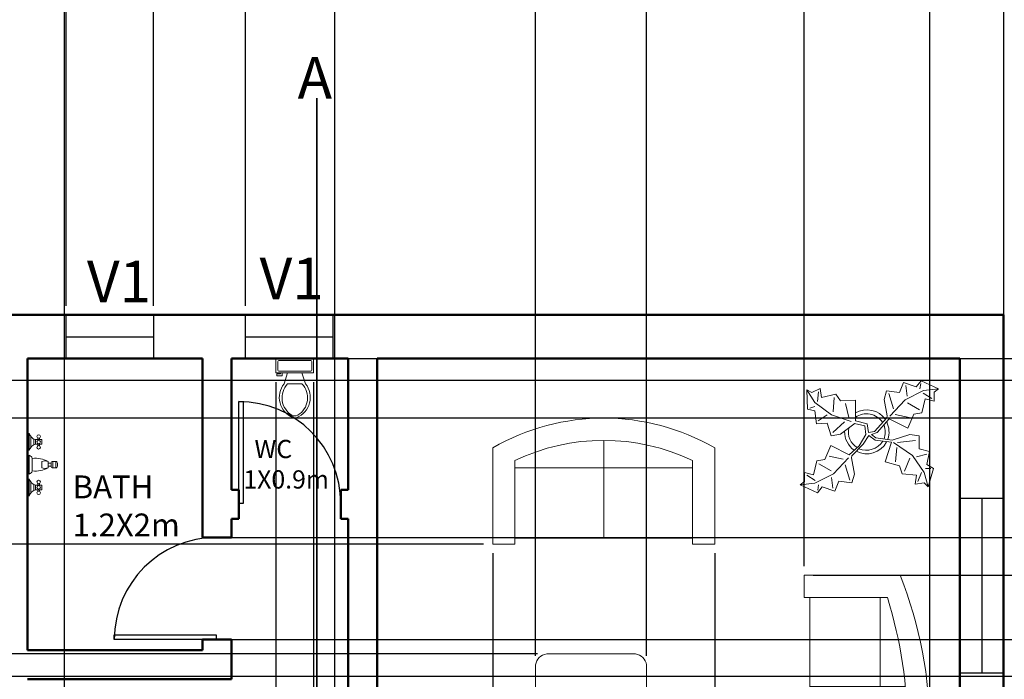
# Model space of a CAD drawing. Units: metres. Extents: x 2443.7 to 2482.9, y 2261.4 to 2287.
# Tile 5 of 8: x 2451.1 to 2457.9, y 2272.3 to 2276.8. Entities that reach past the tile are written whole.
import ezdxf

# ---------------------------------------------------------------- set-up
doc = ezdxf.new("R2010")
doc.units = ezdxf.units.M
for name, color, linetype, lineweight in [('A-ANNO-DIMS', 2, 'Continuous', 18), ('A-AREA-IDEN', 11, 'Continuous', 25), ('A-FLOR-FIXT', 20, 'Continuous', 18), ('A-MODL', 7, 'Continuous', 25), ('A-WALL', 7, 'Continuous', 50), ('door', 6, 'Continuous', 25), ('flower', 70, 'Continuous', 18), ('furnitures', 20, 'Continuous', 18), ('section', 1, 'Continuous', 35), ('text', 11, 'Continuous', 25), ('window', 3, 'Continuous', 25)]:
    doc.layers.add(name, color=color, linetype=linetype, lineweight=lineweight)
doc.styles.get("Standard").update_dxf_attribs({"font": 'arial.ttf'})
doc.dimstyles.get("Standard").update_dxf_attribs({"dimtxt": 0.18, "dimasz": 0.18, "dimexe": 0.18, "dimexo": 0.0625, "dimgap": 0.09, "dimtad": 0, "dimtih": 1, "dimtoh": 1, "dimdec": 4, "dimzin": 0, "dimdsep": 46, "dimtxsty": 'Standard', "dimcen": 0.09, "dimadec": 0, "dimazin": 0, "dimtfac": 1, "dimtdec": 4, "dimtofl": 0, "dimtmove": 0, "dimatfit": 3, "dimfxl": 1, "dimtolj": 1, "dimtzin": 0, "dimarcsym": 0})

# ---------------------------------------------------------------- blocks, each defined once
blk = doc.blocks.new('*U21')
for p, q in [((0, 0), (0, -6)), ((40, 0), (40, -6))]:
    blk.add_line(p, q)
blk.add_lwpolyline([(0, 0), (0, 40), (1.75, 40), (1.75, 0)], close=True)
blk.add_arc((0, 0), 40, 0, 90)
blk = doc.blocks.new('Plant - Rubber or Philodendron')
for p, q in [((8.8871, 10.7908), (9.9809, 13.4933)), ((9.9809, 13.4933), (13.3837, 12.301)), ((13.3837, 12.301), (14.68, 13.9039)), ((14.68, 13.9039), (19.3848, 11.8146)), ((-16.2005, 11.4774), (-13.9899, 8.1064)), ((-16.2005, 11.4774), (-14.8639, 10.7964)), ((-16.0159, 6.3329), (-16.2005, 11.4774)), ((-14.8639, 10.7964), (-12.6195, 11.8975)), ((-13.3174, 8.325), (-13.0735, 11.0065)), ((-12.6195, 11.8975), (-12.1909, 9.4345)), ((4.6914, 8.8812), (5.3859, 11.2828)), ((5.3859, 11.2828), (8.8871, 10.7908)), ((15.3859, 11.3055), (10.3916, 8.7942)), ((10.5828, 12.6946), (10.8893, 9.7953)), ((14.5816, 13.2037), (14.3848, 11.8033)), ((19.3848, 11.8146), (15.3859, 11.3055)), ((19.3848, 11.8146), (18.1868, 10.9119)), ((18.1868, 10.9119), (18.1925, 8.4119)), ((-13.9899, 8.1064), (-9.5434, 4.7185)), ((-12.1909, 9.4345), (-8.3829, 10.3)), ((-8.8369, 9.409), (-9.0894, 5.6095)), ((-8.3829, 10.3), (-7.0549, 8.501)), ((-7.0549, 8.501), (-3.0284, 8.6941)), ((-3.0284, 8.6941), (-3.0709, 3.1041)), ((4.6914, 8.8812), (5.5014, 4.4831)), ((5.9878, 10.4842), (7.1971, 6.3869)), ((10.3916, 8.7942), (6.2847, 4.4028)), ((14.2977, 6.1031), (10.9934, 7.9956)), ((15.7909, 9.1065), (14.8995, 5.3044)), ((15.2875, 10.6053), (17.5907, 9.2105)), ((18.1925, 8.4119), (15.7909, 9.1065)), ((-14.0069, 5.8704), (-16.0159, 6.3329)), ((-15.3434, 6.5514), (-13.9984, 6.9884)), ((-13.5868, 2.2894), (-14.0069, 5.8704)), ((-4.8529, 4.012), (-5.7184, 7.82)), ((-13.1329, 3.1804), (-10.6614, 4.727)), ((-9.5434, 4.7185), (-4.1917, 2.9888)), ((-9.1318, 0.0195), (-5.9793, 2.9025)), ((-3.0709, 3.1041), (0.0797, 2.3163)), ((2.1141, 0.2298), (5.4346, 3.9146)), ((6.1032, 3.6844), (2.8262, -0.031)), ((5.4346, 3.9146), (5.5014, 4.4831)), ((11.1089, 1.1958), (6.1032, 3.6844)), ((7.7005, 4.8881), (11.5025, 3.9967)), ((12.7005, 4.8994), (11.1089, 1.1958)), ((14.8995, 5.3044), (12.7005, 4.8994)), ((-10.6784, 2.491), (-13.5868, 2.2894)), ((-9.5858, -0.8715), (-10.6784, 2.491)), ((-7.1228, -0.443), (-3.5248, 2.2131)), ((-3.5248, 2.2131), (-3.3011, 2.4355)), ((-3.3011, 2.4355), (-0.5306, 1.7947)), ((-0.5306, 1.7947), (-0.2255, -0.5527)), ((-0.5306, 1.7947), (-0.5306, 1.7947)), ((0.0797, 2.3163), (0.4866, -0.031)), ((0.4866, -0.031), (2.1141, 0.2298)), ((-7.1228, -0.443), (-9.5858, -0.8715)), ((-2.019, -3.6148), (-0.2255, -0.5527)), ((-0.9375, -3.1608), (0.5883, -0.8135)), ((0.5883, -0.8135), (2.2447, -2.0916)), ((2.8262, -0.031), (1.3003, -0.5527)), ((1.3003, -0.5527), (2.4193, -1.4655)), ((2.2447, -2.0916), (6.7108, -2.6626)), ((2.4193, -1.4655), (6.895, -2.1175)), ((11.6605, -0.5413), (6.895, -2.1175)), ((8.3544, -2.7453), (13.1973, -2.1704)), ((11.6605, -0.5413), (14.1354, -0.8948)), ((14.1354, -0.8948), (14.1354, -4.4304)), ((-11.3237, -7.2629), (-9.7321, -3.5593)), ((-9.7321, -3.5593), (-4.7264, -6.0479)), ((-2.019, -3.6148), (-4.7264, -6.0479)), ((-4.0579, -6.2781), (-0.9375, -3.1608)), ((4.943, -7.9659), (6.7108, -2.6626)), ((12.3677, -6.1981), (7.219, -2.6772)), ((8.125, -4.0768), (7.7715, -7.9659)), ((14.1354, -4.4304), (16.9638, -5.1375)), ((16.9638, -5.1375), (16.2567, -8.673)), ((-14.4141, -11.4699), (-13.5228, -7.6679)), ((-13.5228, -7.6679), (-11.3237, -7.2629)), ((-6.3237, -7.2516), (-10.1257, -6.3602)), ((-9.0148, -11.1577), (-4.9047, -6.8122)), ((-4.1246, -6.8466), (-4.0579, -6.2781)), ((-3.3146, -11.2447), (-4.1246, -6.8466)), ((8.8321, -9.0266), (4.943, -7.9659)), ((10.2463, -10.4408), (11.6605, -6.9053)), ((15.5496, -10.7943), (12.3677, -6.1981)), ((16.2567, -5.8446), (13.4283, -6.5517)), ((-12.921, -8.4665), (-9.6166, -10.359)), ((-4.611, -12.8477), (-5.8203, -8.7504)), ((9.5392, -11.1479), (8.8321, -9.0266)), ((17.3174, -9.7337), (15.9032, -9.7337)), ((16.2567, -8.673), (18.0245, -9.7337)), ((18.0245, -9.7337), (16.6103, -14.6834)), ((-18.008, -14.1781), (-16.8101, -13.2754)), ((-16.8157, -10.7754), (-14.4141, -11.4699)), ((-16.8101, -13.2754), (-16.8157, -10.7754)), ((-13.9107, -12.9688), (-16.2139, -11.574)), ((-14.0091, -13.669), (-9.0148, -11.1577)), ((-9.206, -15.0581), (-9.5126, -12.1588)), ((-7.5103, -13.1543), (-8.6042, -15.8568)), ((-4.0092, -13.6463), (-7.5103, -13.1543)), ((-3.3146, -11.2447), (-4.0092, -13.6463)), ((13.4283, -11.5015), (9.5392, -11.1479)), ((13.0748, -13.9763), (13.4283, -11.5015)), ((14.8425, -10.7943), (13.7819, -13.2692)), ((16.6103, -14.6834), (15.5496, -10.7943)), ((-18.008, -14.1781), (-14.0091, -13.669)), ((-13.3032, -16.2674), (-18.008, -14.1781)), ((-12.0069, -14.6645), (-13.3032, -16.2674)), ((-13.2048, -15.5672), (-13.008, -14.1668)), ((-8.6042, -15.8568), (-12.0069, -14.6645)), ((15.5496, -13.6228), (13.0748, -13.9763)), ((16.6103, -14.6834), (15.5496, -13.6228))]:
    blk.add_line(p, q)
for centre, radius, start, end in [((0, 0), 6.1275, 34.37569, 120.1028), ((-0.0601, -0.2075), 5.2461, 33.82192, 124.9414), ((-0.098, 0.1364), 6.1288, 341.2017, 26.09184), ((0.0308, 0.1664), 6, 178.6147, 235.1169), ((0.0308, 0.1664), 5, 168.1647, 238.6725), ((-0.2664, 0.1682), 5.2775, 338.4094, 20.03007), ((-0.0234, 0.3825), 6.1492, 242.5812, 331.2714), ((-0.1102, 0.4886), 5.2883, 247.3711, 327.472)]:
    blk.add_arc(centre, radius, start, end)
blk = doc.blocks.new('Sofa - Roundback 7 ft.')
for p, q in [((-12.00002, -32.4421), (-12.00003, -6.5971)), ((11.99997, -32.4421), (11.99998, -6.5971)), ((-36.000027, -34), (-36.000027, -11.4696)), ((35.99998, -34), (35.99998, -11.4696)), ((-35.999844, -13.3819), (35.9998, -13.3819)), ((-36.000027, -32.4421), (35.99998, -32.4421))]:
    blk.add_line(p, q)
for points in [[(-36.000027, -34), (-42.000027, -34), (-42.000027, -8)], [(41.99998, -8), (41.99998, -34), (35.99998, -34)]]:
    blk.add_lwpolyline(points)
for centre, radius, start, end in [((0, -114.25), 114.25, 68.43141, 111.5686), ((-0.00001, -127.1968), 121.1968, 72.72033, 107.2797)]:
    blk.add_arc(centre, radius, start, end)
blk = doc.blocks.new('Sofa - Roundback Loveseat 5 ft.')
for p, q in [((0, -32.44198), (0, -5.99998)), ((-24, -33.99998), (-24, -11.46958)), ((24.00004, -33.99998), (24.00004, -11.46958)), ((-23.9998, -13.38178), (23.99986, -13.38178)), ((-24, -32.44198), (24.00004, -32.44198))]:
    blk.add_line(p, q)
for points in [[(-24, -33.99998), (-30, -33.99998), (-30, -7.99998)], [(30.00004, -7.99998), (30.00004, -33.99998), (24.00004, -33.99998)]]:
    blk.add_lwpolyline(points)
for centre, radius, start, end in [((0, -60.24998), 60.24998, 60.13715, 119.8628), ((0, -61.38438), 55.38444, 64.32083, 115.6792)]:
    blk.add_arc(centre, radius, start, end)
blk = doc.blocks.new('Desk - 30 x 60 in.')
for p, q in [((-26.999995, 0), (26.999995, 0)), ((-29.999995, -27), (-29.999995, -3)), ((29.999995, -3), (29.999995, -27)), ((26.999995, -30), (-26.999995, -30)), ((-20.000005, -30), (-20.000005, -31)), ((-20.000005, -31), (-16.000005, -31)), ((-16.000005, -31), (-16.000005, -30)), ((15.999995, -31), (15.999995, -30)), ((19.999995, -31), (15.999995, -31)), ((19.999995, -30), (19.999995, -31))]:
    blk.add_line(p, q)
for centre, start, end in [((-26.499995, -3.5), 98.1301, 171.8699), ((26.499995, -3.5), 8.130102, 81.8699), ((-26.499995, -26.5), 188.1301, 261.8699), ((26.499995, -26.5), 278.1301, 351.8699)]:
    blk.add_arc(centre, 3.535534, start, end)
blk = doc.blocks.new('Toilet - top')
for p, q in [((9.5, -6), (9.5, -2)), ((-10, -8.5), (-8, -8.5)), ((-10, -9.5), (-10, -8.5)), ((-7, -9.5), (-10, -9.5)), ((-8, -8.5), (-8, -8)), ((-7, -8), (-7, -9.5)), ((-4, -8), (-6, -14)), ((4, -8), (6, -14)), ((4, -14), (-4, -14))]:
    blk.add_line(p, q)
blk.add_lwpolyline([(10.5, -8), (10.5, 0), (-10.5, 0), (-10.5, -8)], close=True)
for points in [[(-9.5, -2), (-9.5, -6)], [(8.5, -1), (-8.5, -1)], [(-8.5, -7), (8.5, -7)]]:
    blk.add_lwpolyline(points)
for centre, radius, start, end in [((-8.62, -1.88), 0.884, 81.8699, 188.1301), ((8.62, -1.88), 0.884, 351.8699, 98.1301), ((-8.62, -6.12), 0.884, 171.8699, 278.1301), ((8.62, -6.12), 0.884, 261.8699, 8.1301), ((3.52, -21.58), 12.17, 141.4691, 247.9714), ((4.2, -21.82), 11.33, 136.3677, 238.9468), ((-3.52, -21.58), 12.17, 292.0284, 38.5307), ((-4.2, -21.82), 11.33, 301.053, 43.6321), ((0, -27.88), 4, 245.7318, 294.2682), ((0, -29), 4, 254.8605, 285.1395)]:
    blk.add_arc(centre, radius, start, end)
blk = doc.blocks.new('Faucet - Bathroom front')
for p, q in [((-0.5, 4.25), (0.5, 4.25)), ((0.5, 3.75), (-0.5, 3.75)), ((-0.25, 3), (-0.25, 3.5)), ((0.25, 3.5), (0.25, 3)), ((-4, 1.625), (-4.25, 1.625)), ((-3.25, 1.625), (-3, 1.625)), ((-0.5, 3), (0.5, 3)), ((0.5, 2), (-0.5, 2)), ((3.25, 1.625), (3, 1.625)), ((4, 1.625), (4.25, 1.625)), ((-5, 0), (-2.25, 0)), ((-4.5087, 0.25), (-2.7408, 0.25)), ((-4, 1.375), (-4.25, 1.375)), ((-3.1442, 0.75), (-4.0979, 0.75)), ((-3.25, 1.375), (-3, 1.375)), ((-1.5, 0), (1.5, 0)), ((-1, 0.5), (1, 0.5)), ((2.25, 0), (5, 0)), ((2.7413, 0.25), (4.5092, 0.25)), ((3.25, 1.375), (3, 1.375)), ((4.1058, 0.75), (3.1521, 0.75)), ((4, 1.375), (4.25, 1.375))]:
    blk.add_line(p, q)
for points in [[(-0.5, 3.75), (-0.5, 4.25)], [(-0.25, 4.5), (0.25, 4.5)], [(0.25, 3.5), (-0.25, 3.5)], [(0.5, 4.25), (0.5, 3.75)]]:
    blk.add_lwpolyline(points)
for points in [[(-4, 1), (-4, 2), (-3.25, 2), (-3.25, 1)], [(3.25, 1), (3.25, 2), (4, 2), (4, 1)]]:
    blk.add_lwpolyline(points, close=True)
for centre in [(-4.5, 1.5), (-3.625, 1.5), (-2.75, 1.5), (2.75, 1.5), (3.625, 1.5), (4.5, 1.5)]:
    blk.add_circle(centre, 0.2795)
for centre, radius, start, end in [((-0.2575, 4.2575), 0.2426, 88.22243, 181.7776), ((-0.2575, 3.7425), 0.2426, 178.2224, 271.7776), ((0.2575, 4.2575), 0.2426, 358.2224, 91.77757), ((0.2575, 3.7425), 0.2426, 268.2224, 1.777565), ((3, 1), 4.0311, 150.2551, 187.125), ((0.6413, 2.5), 1.246, 156.3417, 203.6583), ((-3, 1), 4.0311, 352.875, 29.74488), ((-0.6413, 2.5), 1.246, 336.3417, 23.65835), ((-5.375, 1.375), 1.4252, 285.2551, 344.7449), ((-1.875, 1.375), 1.4252, 195.2551, 254.7449), ((-0.7962, -0.2038), 0.7327, 106.1502, 163.8498), ((0.7962, -0.2038), 0.7327, 16.1502, 73.84979), ((1.875, 1.375), 1.4252, 285.2551, 344.7449), ((5.375, 1.375), 1.4252, 195.2551, 254.7449)]:
    blk.add_arc(centre, radius, start, end)
blk = doc.blocks.new('aditya')
at = {"layer": 'A-WALL'}
for p, q in [((0, 9.9), (10.2, 9.9)), ((10.2, 3.3), (10.2, 9.9)), ((3.5, 7.6), (3.5, 9.6)), ((3.5, 9.6), (4.7, 9.6)), ((4.7, 8.3734), (4.7, 9.6)), ((4.9, 8.7), (4.9, 9.6)), ((4.9, 9.6), (5.7, 9.6)), ((5.7, 8.7), (5.7, 9.6)), ((5.9, 6.0521), (5.9, 9.6)), ((5.9, 9.6), (9.9, 9.6)), ((9.9, 5), (9.9, 9.6)), ((4.9, 8.7), (4.9503, 8.7)), ((5.6503, 8.7), (5.7, 8.7)), ((4.9, 8.3734), (4.9, 8.5)), ((4.9, 8.5), (4.9503, 8.5)), ((5.6503, 8.5), (5.7, 8.5)), ((5.7, 6.0521), (5.7, 8.5)), ((4.7, 7.6), (4.7, 7.6734)), ((4.9, 7.4), (4.9, 7.6734)), ((3.5, 7.6), (4.7, 7.6)), ((3.5, 7.4), (4.9, 7.4))]:
    blk.add_line(p, q, dxfattribs=at)
for points in [[(4.9503, 8.5), (4.9503, 8.7)], [(5.6503, 8.7), (5.6503, 8.5)], [(4.7, 8.3734), (4.9, 8.3734)], [(4.9, 7.6734), (4.7, 7.6734)]]:
    blk.add_lwpolyline(points, dxfattribs=at)
at = {"layer": 'section'}
blk.add_line((5.4866, -1.5581), (5.4866, 11.3875), dxfattribs=at)
at = {"layer": 'window'}
for p, q in [((3.7644, 9.75), (4.3644, 9.75)), ((4.9948, 9.75), (5.5948, 9.75)), ((10.05, 8.642), (10.05, 7.442))]:
    blk.add_line(p, q, dxfattribs=at)
for points in [[(3.7644, 9.6), (3.7644, 9.9), (4.3644, 9.9), (4.3644, 9.6)], [(4.9948, 9.6), (4.9948, 9.9), (5.5948, 9.9), (5.5948, 9.6)], [(9.9, 8.642), (10.2, 8.642), (10.2, 7.442), (9.9, 7.442)]]:
    blk.add_lwpolyline(points, close=True, dxfattribs=at)
at = {"layer": 'A-FLOR-FIXT', "xscale": 0.0123151634342974, "yscale": 0.0123151634342974, "zscale": 0.0123151634342974}
blk.add_blockref('Toilet - top', (5.3344, 9.6), dxfattribs=at)
at = {"layer": 'A-FLOR-FIXT', "xscale": 0.0430474379416969, "yscale": 0.0430474379416969, "zscale": 0.0430474379416969, "rotation": 270}
blk.add_blockref('Faucet - Bathroom front', (3.511, 8.8725), dxfattribs=at)
at = {"layer": 'door', "xscale": 0.0174999999999987, "yscale": 0.0174999999999987, "zscale": 0.0174999999999987}
blk.add_blockref('*U21', (4.9503, 8.605), dxfattribs=at)
at = {"layer": 'door', "xscale": 0.0174999999999987, "yscale": 0.0174999999999987, "zscale": 0.0174999999999987, "rotation": 90}
blk.add_blockref('*U21', (4.795, 7.6734), dxfattribs=at)
at = {"layer": 'flower', "xscale": 0.0254, "yscale": 0.0254, "zscale": 0.0254}
blk.add_blockref('Plant - Rubber or Philodendron', (9.2606, 9.0935), dxfattribs=at)
at = {"layer": 'furnitures', "xscale": 0.0254, "yscale": 0.0254, "zscale": 0.0254}
blk.add_blockref('Sofa - Roundback Loveseat 5 ft.', (7.4549, 9.1917), dxfattribs=at)
for name, p, rotation in [('Sofa - Roundback 7 ft.', (9.6938, 7.0466), 270), ('Desk - 30 x 60 in.', (6.9873, 6.8124), 90)]:
    blk.add_blockref(name, p, dxfattribs=dict(at, rotation=rotation))
at = {"layer": 'A-AREA-IDEN', "attachment_point": 1}
for s, width, gutter_width, insert, char_height in [('{\\fArial|b1|i1|c0|p34;  WC\\P1X0.9m}', 5.273298, 3.9123, (4.9809, 9.0426), 0.125192), ('{\\fArial|b1|i1|c0|p34;BATH\\P1.2X2m}', 6.599358, 4.8961, (3.8093, 8.7984), 0.156674)]:
    blk.add_mtext_dynamic_manual_height_columns(s, width=width, gutter_width=gutter_width, heights=[0], dxfattribs=dict(at, insert=insert, char_height=char_height))
at = {"layer": 'text'}
for s, height, p in [('A', 0.2853, (5.3535, 11.3838)), ('V1', 0.28528, (5.0929, 10.0065)), ('V1', 0.28528, (3.9077, 9.9863))]:
    blk.add_text(s, height=height, dxfattribs=at).set_placement(p)
blk = doc.blocks.new('*D23')
at = {"layer": 'A-ANNO-DIMS', "color": 0, "lineweight": -2, "transparency": 16777216}
for p, q in [((2457.9453, 2274.7597), (2482.2428, 2274.7597)), ((2482.0628, 2274.5797), (2482.0628, 2269.6416)), ((2482.0628, 2264.3397), (2482.0628, 2269.2778)), ((2453.6453, 2264.1597), (2482.2428, 2264.1597))]:
    blk.add_line(p, q, dxfattribs=at)
at = {"layer": 'A-ANNO-DIMS', "color": 0, "transparency": 16777216}
for points in [[(2482.0328, 2274.5797), (2482.0928, 2274.5797), (2482.0628, 2274.7597)], [(2482.0328, 2264.3397), (2482.0928, 2264.3397), (2482.0628, 2264.1597)]]:
    blk.add_solid(points, dxfattribs=at)
at = {"layer": 'Defpoints', "color": 0, "transparency": 16777216}
for p in [(2457.8828, 2274.7597), (2453.5828, 2264.1597), (2482.0628, 2264.1597)]:
    blk.add_point(p, dxfattribs=at)
at = {"layer": 'A-ANNO-DIMS', "color": 0, "transparency": 16777216, "insert": (2482.0628, 2269.4597), "char_height": 0.18, "attachment_point": 5}
blk.add_mtext('\\A1;10.6', dxfattribs=at)
blk = doc.blocks.new('*D28')
at = {"layer": 'A-ANNO-DIMS', "color": 0, "lineweight": -2, "transparency": 16777216}
for p, q in [((2449.9171, 2274.8222), (2449.9171, 2287.0152)), ((2451.4471, 2274.8222), (2451.4471, 2287.0152)), ((2450.0971, 2286.8352), (2450.3668, 2286.8352)), ((2451.2671, 2286.8352), (2450.9974, 2286.8352))]:
    blk.add_line(p, q, dxfattribs=at)
at = {"layer": 'A-ANNO-DIMS', "color": 0, "transparency": 16777216}
for points in [[(2450.0971, 2286.8652), (2450.0971, 2286.8052), (2449.9171, 2286.8352)], [(2451.2671, 2286.8652), (2451.2671, 2286.8052), (2451.4471, 2286.8352)]]:
    blk.add_solid(points, dxfattribs=at)
at = {"layer": 'Defpoints', "color": 0, "transparency": 16777216}
for p in [(2451.4471, 2286.8352), (2449.9171, 2274.7597), (2451.4471, 2274.7597)]:
    blk.add_point(p, dxfattribs=at)
at = {"layer": 'A-ANNO-DIMS', "color": 0, "transparency": 16777216, "insert": (2450.6821, 2286.8352), "char_height": 0.18, "attachment_point": 5}
blk.add_mtext('\\A1;1.53', dxfattribs=at)
blk = doc.blocks.new('*D29')
at = {"layer": 'A-ANNO-DIMS', "color": 0, "lineweight": -2, "transparency": 16777216}
for p, q in [((2451.4471, 2274.8222), (2451.4471, 2287.0152)), ((2452.0471, 2274.8222), (2452.0471, 2287.0152)), ((2451.6271, 2286.8352), (2451.8671, 2286.8352)), ((2452.0471, 2286.8352), (2452.2271, 2286.8352))]:
    blk.add_line(p, q, dxfattribs=at)
at = {"layer": 'A-ANNO-DIMS', "color": 0, "transparency": 16777216}
for points in [[(2451.6271, 2286.8652), (2451.6271, 2286.8052), (2451.4471, 2286.8352)], [(2451.8671, 2286.8652), (2451.8671, 2286.8052), (2452.0471, 2286.8352)]]:
    blk.add_solid(points, dxfattribs=at)
at = {"layer": 'Defpoints', "color": 0, "transparency": 16777216}
for p in [(2452.0471, 2286.8352), (2451.4471, 2274.7597), (2452.0471, 2274.7597)]:
    blk.add_point(p, dxfattribs=at)
at = {"layer": 'A-ANNO-DIMS', "color": 0, "transparency": 16777216, "insert": (2452.4809, 2286.8352), "char_height": 0.18, "attachment_point": 5}
blk.add_mtext('\\A1;0.6', dxfattribs=at)
blk = doc.blocks.new('*D30')
at = {"layer": 'A-ANNO-DIMS', "color": 0, "lineweight": -2, "transparency": 16777216}
for p, q in [((2452.0471, 2274.8222), (2452.0471, 2287.0152)), ((2452.6776, 2274.8222), (2452.6776, 2287.0152)), ((2452.2271, 2286.8352), (2452.4976, 2286.8352)), ((2452.6776, 2286.8352), (2452.8576, 2286.8352))]:
    blk.add_line(p, q, dxfattribs=at)
at = {"layer": 'A-ANNO-DIMS', "color": 0, "transparency": 16777216}
for points in [[(2452.2271, 2286.8652), (2452.2271, 2286.8052), (2452.0471, 2286.8352)], [(2452.4976, 2286.8652), (2452.4976, 2286.8052), (2452.6776, 2286.8352)]]:
    blk.add_solid(points, dxfattribs=at)
at = {"layer": 'Defpoints', "color": 0, "transparency": 16777216}
for p in [(2452.6776, 2286.8352), (2452.0471, 2274.7597), (2452.6776, 2274.7597)]:
    blk.add_point(p, dxfattribs=at)
at = {"layer": 'A-ANNO-DIMS', "color": 0, "transparency": 16777216, "insert": (2453.1813, 2286.8352), "char_height": 0.18, "attachment_point": 5}
blk.add_mtext('\\A1;0.63', dxfattribs=at)
blk = doc.blocks.new('*D34')
at = {"layer": 'A-ANNO-DIMS', "color": 0, "lineweight": -2, "transparency": 16777216}
for p, q in [((2457.9453, 2274.7597), (2482.2428, 2274.7597)), ((2482.0628, 2274.5797), (2482.0628, 2274.3126)), ((2482.0628, 2273.6817), (2482.0628, 2273.9488)), ((2457.9453, 2273.5017), (2482.2428, 2273.5017))]:
    blk.add_line(p, q, dxfattribs=at)
at = {"layer": 'A-ANNO-DIMS', "color": 0, "transparency": 16777216}
for points in [[(2482.0328, 2274.5797), (2482.0928, 2274.5797), (2482.0628, 2274.7597)], [(2482.0328, 2273.6817), (2482.0928, 2273.6817), (2482.0628, 2273.5017)]]:
    blk.add_solid(points, dxfattribs=at)
at = {"layer": 'Defpoints', "color": 0, "transparency": 16777216}
for p in [(2457.8828, 2274.7597), (2457.8828, 2273.5017), (2482.0628, 2273.5017)]:
    blk.add_point(p, dxfattribs=at)
at = {"layer": 'A-ANNO-DIMS', "color": 0, "transparency": 16777216, "insert": (2482.0628, 2274.1307), "char_height": 0.18, "attachment_point": 5}
blk.add_mtext('\\A1;1.258', dxfattribs=at)
blk = doc.blocks.new('*D35')
at = {"layer": 'A-ANNO-DIMS', "color": 0, "lineweight": -2, "transparency": 16777216}
for p, q in [((2457.9453, 2272.3017), (2482.2428, 2272.3017)), ((2482.0628, 2272.1217), (2482.0628, 2271.6247)), ((2482.0628, 2270.7669), (2482.0628, 2271.2639)), ((2457.9453, 2270.5869), (2482.2428, 2270.5869))]:
    blk.add_line(p, q, dxfattribs=at)
at = {"layer": 'A-ANNO-DIMS', "color": 0, "transparency": 16777216}
for points in [[(2482.0328, 2272.1217), (2482.0928, 2272.1217), (2482.0628, 2272.3017)], [(2482.0328, 2270.7669), (2482.0928, 2270.7669), (2482.0628, 2270.5869)]]:
    blk.add_solid(points, dxfattribs=at)
at = {"layer": 'Defpoints', "color": 0, "transparency": 16777216}
for p in [(2457.8828, 2272.3017), (2457.8828, 2270.5869), (2482.0628, 2270.5869)]:
    blk.add_point(p, dxfattribs=at)
at = {"layer": 'A-ANNO-DIMS', "color": 0, "transparency": 16777216, "insert": (2482.0628, 2271.4443), "char_height": 0.18, "attachment_point": 5}
blk.add_mtext('\\A1;1.71', dxfattribs=at)
blk = doc.blocks.new('*D37')
at = {"layer": 'A-ANNO-DIMS', "color": 0, "lineweight": -2, "transparency": 16777216}
for p, q in [((2450.1874, 2274.3123), (2482.2428, 2274.3123)), ((2482.0628, 2274.1323), (2482.0628, 2273.4783)), ((2482.0628, 2272.4603), (2482.0628, 2273.1144)), ((2450.1874, 2272.2803), (2482.2428, 2272.2803))]:
    blk.add_line(p, q, dxfattribs=at)
at = {"layer": 'A-ANNO-DIMS', "color": 0, "transparency": 16777216}
for points in [[(2482.0328, 2274.1323), (2482.0928, 2274.1323), (2482.0628, 2274.3123)], [(2482.0328, 2272.4603), (2482.0928, 2272.4603), (2482.0628, 2272.2803)]]:
    blk.add_solid(points, dxfattribs=at)
at = {"layer": 'Defpoints', "color": 0, "transparency": 16777216}
for p in [(2450.1249, 2274.3123), (2482.0628, 2274.3123), (2450.1249, 2272.2803)]:
    blk.add_point(p, dxfattribs=at)
at = {"layer": 'A-ANNO-DIMS', "color": 0, "transparency": 16777216, "insert": (2482.0628, 2273.2963), "char_height": 0.18, "attachment_point": 5}
blk.add_mtext('\\A1;2.032', dxfattribs=at)
blk = doc.blocks.new('*D38')
at = {"layer": 'A-ANNO-DIMS', "color": 0, "lineweight": -2, "transparency": 16777216}
for p, q in [((2454.3757, 2273.1253), (2454.3757, 2261.3876)), ((2455.8997, 2273.1253), (2455.8997, 2261.3876)), ((2454.5557, 2261.5676), (2454.7528, 2261.5676)), ((2455.7197, 2261.5676), (2455.5225, 2261.5676))]:
    blk.add_line(p, q, dxfattribs=at)
at = {"layer": 'A-ANNO-DIMS', "color": 0, "transparency": 16777216}
for points in [[(2454.5557, 2261.5976), (2454.5557, 2261.5376), (2454.3757, 2261.5676)], [(2455.7197, 2261.5976), (2455.7197, 2261.5376), (2455.8997, 2261.5676)]]:
    blk.add_solid(points, dxfattribs=at)
at = {"layer": 'Defpoints', "color": 0, "transparency": 16777216}
for p in [(2454.3757, 2273.1878), (2455.8997, 2273.1878), (2454.3757, 2261.5676)]:
    blk.add_point(p, dxfattribs=at)
at = {"layer": 'A-ANNO-DIMS', "color": 0, "transparency": 16777216, "insert": (2455.1377, 2261.5676), "char_height": 0.18, "attachment_point": 5}
blk.add_mtext('\\A1;1.524', dxfattribs=at)
blk = doc.blocks.new('*D39')
at = {"layer": 'A-ANNO-DIMS', "color": 0, "lineweight": -2, "transparency": 16777216}
for p, q in [((2444.2827, 2274.0514), (2444.2827, 2274.2314)), ((2444.2827, 2274.2314), (2444.4627, 2274.2314)), ((2455.0752, 2274.0514), (2444.1027, 2274.0514)), ((2444.2827, 2273.3678), (2444.2827, 2273.8714)), ((2454.3132, 2273.1878), (2444.1027, 2273.1878))]:
    blk.add_line(p, q, dxfattribs=at)
at = {"layer": 'A-ANNO-DIMS', "color": 0, "transparency": 16777216}
for points in [[(2444.2527, 2273.8714), (2444.3127, 2273.8714), (2444.2827, 2274.0514)], [(2444.2527, 2273.3678), (2444.3127, 2273.3678), (2444.2827, 2273.1878)]]:
    blk.add_solid(points, dxfattribs=at)
at = {"layer": 'Defpoints', "color": 0, "transparency": 16777216}
for p in [(2444.2827, 2274.0514), (2455.1377, 2274.0514), (2454.3757, 2273.1878)]:
    blk.add_point(p, dxfattribs=at)
at = {"layer": 'A-ANNO-DIMS', "color": 0, "transparency": 16777216, "insert": (2444.7864, 2274.2314), "char_height": 0.18, "attachment_point": 5}
blk.add_mtext('\\A1;0.86', dxfattribs=at)
blk = doc.blocks.new('*D40')
at = {"layer": 'A-ANNO-DIMS', "color": 0, "lineweight": -2, "transparency": 16777216}
for p, q in [((2456.5754, 2272.973), (2482.2428, 2272.973)), ((2482.0628, 2272.793), (2482.0628, 2272.0882)), ((2482.0628, 2271.0194), (2482.0628, 2271.7243)), ((2456.5754, 2270.8394), (2482.2428, 2270.8394))]:
    blk.add_line(p, q, dxfattribs=at)
at = {"layer": 'A-ANNO-DIMS', "color": 0, "transparency": 16777216}
for points in [[(2482.0328, 2272.793), (2482.0928, 2272.793), (2482.0628, 2272.973)], [(2482.0328, 2271.0194), (2482.0928, 2271.0194), (2482.0628, 2270.8394)]]:
    blk.add_solid(points, dxfattribs=at)
at = {"layer": 'Defpoints', "color": 0, "transparency": 16777216}
for p in [(2456.5129, 2272.973), (2482.0628, 2272.973), (2456.5129, 2270.8394)]:
    blk.add_point(p, dxfattribs=at)
at = {"layer": 'A-ANNO-DIMS', "color": 0, "transparency": 16777216, "insert": (2482.0628, 2271.9062), "char_height": 0.18, "attachment_point": 5}
blk.add_mtext('\\A1;2.13', dxfattribs=at)
blk = doc.blocks.new('*D41')
at = {"layer": 'A-ANNO-DIMS', "color": 0, "lineweight": -2, "transparency": 16777216}
for p, q in [((2456.512931, 2273.035548), (2456.512931, 2287.015188)), ((2457.376531, 2271.968748), (2457.376531, 2287.015188)), ((2456.332931, 2286.835188), (2456.152931, 2286.835188)), ((2457.556531, 2286.835188), (2457.736531, 2286.835188))]:
    blk.add_line(p, q, dxfattribs=at)
at = {"layer": 'A-ANNO-DIMS', "color": 0, "transparency": 16777216}
for points in [[(2456.332931, 2286.865188), (2456.332931, 2286.805188), (2456.512931, 2286.835188)], [(2457.556531, 2286.865188), (2457.556531, 2286.805188), (2457.376531, 2286.835188)]]:
    blk.add_solid(points, dxfattribs=at)
at = {"layer": 'Defpoints', "color": 0, "transparency": 16777216}
for p in [(2457.376531, 2286.835188), (2456.512931, 2272.973048), (2457.376531, 2271.906248)]:
    blk.add_point(p, dxfattribs=at)
at = {"layer": 'A-ANNO-DIMS', "color": 0, "transparency": 16777216, "insert": (2456.944731, 2286.835188), "char_height": 0.18, "attachment_point": 5}
blk.add_mtext('\\A1;0.86', dxfattribs=at)
blk = doc.blocks.new('*D42')
at = {"layer": 'A-ANNO-DIMS', "color": 0, "lineweight": -2, "transparency": 16777216}
for p, q in [((2454.6838, 2272.434), (2444.1027, 2272.434)), ((2444.2827, 2272.254), (2444.2827, 2271.854)), ((2444.2827, 2271.09), (2444.2827, 2271.4901)), ((2454.6838, 2270.91), (2444.1027, 2270.91))]:
    blk.add_line(p, q, dxfattribs=at)
at = {"layer": 'A-ANNO-DIMS', "color": 0, "transparency": 16777216}
for points in [[(2444.2527, 2272.254), (2444.3127, 2272.254), (2444.2827, 2272.434)], [(2444.2527, 2271.09), (2444.3127, 2271.09), (2444.2827, 2270.91)]]:
    blk.add_solid(points, dxfattribs=at)
at = {"layer": 'Defpoints', "color": 0, "transparency": 16777216}
for p in [(2444.2827, 2272.434), (2454.7463, 2272.434), (2454.7463, 2270.91)]:
    blk.add_point(p, dxfattribs=at)
at = {"layer": 'A-ANNO-DIMS', "color": 0, "transparency": 16777216, "insert": (2444.2827, 2271.672), "char_height": 0.18, "attachment_point": 5}
blk.add_mtext('\\A1;1.524', dxfattribs=at)
blk = doc.blocks.new('*D43')
at = {"layer": 'A-ANNO-DIMS', "color": 0, "lineweight": -2, "transparency": 16777216}
for p, q in [((2454.6701, 2272.4203), (2454.6701, 2287.0152)), ((2455.4321, 2272.4203), (2455.4321, 2287.0152)), ((2454.8501, 2286.8352), (2455.2521, 2286.8352)), ((2455.4321, 2286.8352), (2455.6121, 2286.8352))]:
    blk.add_line(p, q, dxfattribs=at)
at = {"layer": 'A-ANNO-DIMS', "color": 0, "transparency": 16777216}
for points in [[(2454.8501, 2286.8652), (2454.8501, 2286.8052), (2454.6701, 2286.8352)], [(2455.2521, 2286.8652), (2455.2521, 2286.8052), (2455.4321, 2286.8352)]]:
    blk.add_solid(points, dxfattribs=at)
at = {"layer": 'Defpoints', "color": 0, "transparency": 16777216}
for p in [(2455.4321, 2286.8352), (2454.6701, 2272.3578), (2455.4321, 2272.3578)]:
    blk.add_point(p, dxfattribs=at)
at = {"layer": 'A-ANNO-DIMS', "color": 0, "transparency": 16777216, "insert": (2456.0048, 2286.8352), "char_height": 0.18, "attachment_point": 5}
blk.add_mtext('\\A1;0.762', dxfattribs=at)
blk = doc.blocks.new('*D54')
at = {"layer": 'A-ANNO-DIMS', "color": 0, "lineweight": -2, "transparency": 16777216}
for p, q in [((2482.0628, 2273.2331), (2482.0628, 2273.4131)), ((2482.0628, 2273.4131), (2482.2428, 2273.4131)), ((2452.5403, 2273.2331), (2482.2428, 2273.2331)), ((2482.0628, 2272.7131), (2482.0628, 2273.0531)), ((2452.5403, 2272.5331), (2482.2428, 2272.5331))]:
    blk.add_line(p, q, dxfattribs=at)
at = {"layer": 'A-ANNO-DIMS', "color": 0, "transparency": 16777216}
for points in [[(2482.0328, 2273.0531), (2482.0928, 2273.0531), (2482.0628, 2273.2331)], [(2482.0328, 2272.7131), (2482.0928, 2272.7131), (2482.0628, 2272.5331)]]:
    blk.add_solid(points, dxfattribs=at)
at = {"layer": 'Defpoints', "color": 0, "transparency": 16777216}
for p in [(2452.4778, 2273.2331), (2482.0628, 2273.2331), (2452.4778, 2272.5331)]:
    blk.add_point(p, dxfattribs=at)
at = {"layer": 'A-ANNO-DIMS', "color": 0, "transparency": 16777216, "insert": (2482.4966, 2273.4131), "char_height": 0.18, "attachment_point": 5}
blk.add_mtext('\\A1;0.7', dxfattribs=at)
blk = doc.blocks.new('*D55')
at = {"layer": 'A-ANNO-DIMS', "color": 0, "lineweight": -2, "transparency": 16777216}
for p, q in [((2452.8879, 2274.2987), (2452.8879, 2261.3876)), ((2453.1465, 2274.2987), (2453.1465, 2261.3876)), ((2452.7079, 2261.5676), (2452.5279, 2261.5676)), ((2453.3265, 2261.5676), (2453.5065, 2261.5676))]:
    blk.add_line(p, q, dxfattribs=at)
at = {"layer": 'A-ANNO-DIMS', "color": 0, "transparency": 16777216}
for points in [[(2452.7079, 2261.5976), (2452.7079, 2261.5376), (2452.8879, 2261.5676)], [(2453.3265, 2261.5976), (2453.3265, 2261.5376), (2453.1465, 2261.5676)]]:
    blk.add_solid(points, dxfattribs=at)
at = {"layer": 'Defpoints', "color": 0, "transparency": 16777216}
for p in [(2452.8879, 2274.3612), (2453.1465, 2274.3612), (2453.1465, 2261.5676)]:
    blk.add_point(p, dxfattribs=at)
at = {"layer": 'A-ANNO-DIMS', "color": 0, "transparency": 16777216, "insert": (2453.8302, 2261.5676), "char_height": 0.18, "attachment_point": 5}
blk.add_mtext('\\A1;0.26', dxfattribs=at)
blk = doc.blocks.new('*D56')
at = {"layer": 'A-ANNO-DIMS', "color": 0, "lineweight": -2, "transparency": 16777216}
for p, q in [((2482.062768, 2274.639673), (2482.062768, 2274.819673)), ((2453.208999, 2274.459673), (2482.242768, 2274.459673)), ((2453.07969, 2274.053273), (2482.242768, 2274.053273)), ((2482.062768, 2273.873273), (2482.062768, 2273.693273))]:
    blk.add_line(p, q, dxfattribs=at)
at = {"layer": 'A-ANNO-DIMS', "color": 0, "transparency": 16777216}
for points in [[(2482.032768, 2274.639673), (2482.092768, 2274.639673), (2482.062768, 2274.459673)], [(2482.032768, 2273.873273), (2482.092768, 2273.873273), (2482.062768, 2274.053273)]]:
    blk.add_solid(points, dxfattribs=at)
at = {"layer": 'Defpoints', "color": 0, "transparency": 16777216}
for p in [(2453.146499, 2274.459673), (2482.062768, 2274.459673), (2453.01719, 2274.053273)]:
    blk.add_point(p, dxfattribs=at)
at = {"layer": 'A-ANNO-DIMS', "color": 0, "transparency": 16777216, "insert": (2482.062768, 2274.256473), "char_height": 0.18, "attachment_point": 5}
blk.add_mtext('\\A1;0.41', dxfattribs=at)
blk = doc.blocks.new('*D63')
at = {"layer": 'A-ANNO-DIMS', "color": 0, "lineweight": -2, "transparency": 16777216}
for p, q in [((2447.6828, 2278.9987), (2447.6828, 2261.3876)), ((2457.8828, 2278.9987), (2457.8828, 2261.3876)), ((2447.8628, 2261.5676), (2452.4684, 2261.5676)), ((2457.7028, 2261.5676), (2453.0971, 2261.5676))]:
    blk.add_line(p, q, dxfattribs=at)
at = {"layer": 'A-ANNO-DIMS', "color": 0, "transparency": 16777216}
for points in [[(2447.8628, 2261.5976), (2447.8628, 2261.5376), (2447.6828, 2261.5676)], [(2457.7028, 2261.5976), (2457.7028, 2261.5376), (2457.8828, 2261.5676)]]:
    blk.add_solid(points, dxfattribs=at)
at = {"layer": 'Defpoints', "color": 0, "transparency": 16777216}
for p in [(2447.6828, 2279.0612), (2457.8828, 2279.0612), (2457.8828, 2261.5676)]:
    blk.add_point(p, dxfattribs=at)
at = {"layer": 'A-ANNO-DIMS', "color": 0, "transparency": 16777216, "insert": (2452.7828, 2261.5676), "char_height": 0.18, "attachment_point": 5}
blk.add_mtext('\\A1;10.2', dxfattribs=at)
blk = doc.blocks.new('*D71')
at = {"layer": 'A-ANNO-DIMS', "color": 0, "lineweight": -2, "transparency": 16777216}
for p, q in [((2451.4341, 2281.6186), (2451.4341, 2261.3876)), ((2453.2904, 2281.6186), (2453.2904, 2261.3876)), ((2451.6141, 2261.5676), (2452.047, 2261.5676)), ((2453.1104, 2261.5676), (2452.6775, 2261.5676))]:
    blk.add_line(p, q, dxfattribs=at)
at = {"layer": 'A-ANNO-DIMS', "color": 0, "transparency": 16777216}
for points in [[(2451.6141, 2261.5976), (2451.6141, 2261.5376), (2451.4341, 2261.5676)], [(2453.1104, 2261.5976), (2453.1104, 2261.5376), (2453.2904, 2261.5676)]]:
    blk.add_solid(points, dxfattribs=at)
at = {"layer": 'Defpoints', "color": 0, "transparency": 16777216}
for p in [(2451.4341, 2281.6811), (2453.2904, 2281.6811), (2453.2904, 2261.5676)]:
    blk.add_point(p, dxfattribs=at)
at = {"layer": 'A-ANNO-DIMS', "color": 0, "transparency": 16777216, "insert": (2452.3623, 2261.5676), "char_height": 0.18, "attachment_point": 5}
blk.add_mtext('\\A1;1.86', dxfattribs=at)

msp = doc.modelspace()

# ---------------------------------------------------------------- block references
at = {"layer": 'A-MODL'}
msp.add_blockref('aditya', (2447.682762, 2264.859673), dxfattribs=at)

# ---------------------------------------------------------------- dimensions: what is measured, and where the dimension line sits
at = {"layer": 'A-ANNO-DIMS'}
for base, p1, p2, override, picture, middle in [((2451.44713, 2286.835188), (2449.917083, 2274.759673), (2451.44713, 2274.759673), {"dimdec": 2, "dimlfac": 1, "dimrnd": 0, "dimzin": 0, "dimdsep": 46, "dimlunit": 2}, '*D28', (2450.682106, 2286.835188)), ((2452.04713, 2286.835188), (2451.44713, 2274.759673), (2452.04713, 2274.759673), {"dimdec": 1, "dimlfac": 1, "dimrnd": 0, "dimzin": 0, "dimdsep": 46, "dimlunit": 2}, '*D29', (2452.480923, 2286.835188)), ((2452.677571, 2286.835188), (2452.04713, 2274.759673), (2452.677571, 2274.759673), {"dimdec": 2, "dimlfac": 1, "dimrnd": 0, "dimzin": 0, "dimdsep": 46, "dimlunit": 2}, '*D30', (2453.18135, 2286.835188)), ((2455.432053, 2286.835188), (2454.670053, 2272.357847), (2455.432053, 2272.357847), {"dimdec": 3, "dimlfac": 1, "dimrnd": 0, "dimzin": 0, "dimdsep": 46, "dimlunit": 2}, '*D43', (2456.004836, 2286.835188)), ((2457.376531, 2286.835188), (2456.512931, 2272.973048), (2457.376531, 2271.906248), {"dimdec": 2, "dimlfac": 1, "dimrnd": 0, "dimzin": 0, "dimdsep": 46, "dimlunit": 2}, '*D41', (2456.944731, 2286.835188)), ((2453.29044, 2261.567605), (2451.43413, 2281.681077), (2453.29044, 2281.681077), {"dimdec": 2, "dimlfac": 1, "dimrnd": 0, "dimzin": 0, "dimdsep": 46, "dimlunit": 2}, '*D71', (2452.362285, 2261.567605)), ((2457.882762, 2261.567605), (2447.682762, 2279.061188), (2457.882762, 2279.061188), {"dimdec": 1, "dimlfac": 1, "dimrnd": 0, "dimzin": 0, "dimdsep": 46, "dimlunit": 2}, '*D63', (2452.782762, 2261.567605)), ((2453.146499, 2261.567605), (2452.887881, 2274.361152), (2453.146499, 2274.361152), {"dimdec": 2, "dimlfac": 1, "dimrnd": 0, "dimzin": 0, "dimdsep": 46, "dimlunit": 2}, '*D55', (2453.830217, 2261.567605)), ((2454.375659, 2261.567605), (2455.89966, 2273.187816), (2454.375659, 2273.187816), {"dimdec": 3, "dimlfac": 1, "dimrnd": 0, "dimzin": 0, "dimdsep": 46, "dimlunit": 2}, '*D38', (2455.13766, 2261.567605))]:
    dim = msp.add_linear_dim(base=base, p1=p1, p2=p2, dimstyle='Standard', override=override, dxfattribs=at)
    dim.commit()
    dim.dimension.update_dxf_attribs({"geometry": picture, "text_midpoint": middle})
for base, p1, p2, override, picture, middle in [((2482.062768, 2274.459673), (2453.01719, 2274.053273), (2453.146499, 2274.459673), {"dimdec": 2, "dimlfac": 1, "dimrnd": 0, "dimzin": 0, "dimdsep": 46, "dimlunit": 2}, '*D56', (2482.062768, 2274.256473)), ((2482.062768, 2264.159673), (2457.882762, 2274.759673), (2453.582762, 2264.159673), {"dimdec": 1, "dimlfac": 1, "dimrnd": 0, "dimzin": 0, "dimdsep": 46, "dimlunit": 2}, '*D23', (2482.062768, 2269.459673)), ((2482.062768, 2273.501681), (2457.882762, 2274.759673), (2457.882762, 2273.501681), {"dimdec": 3, "dimlfac": 1, "dimrnd": 0, "dimzin": 0, "dimdsep": 46, "dimlunit": 2}, '*D34', (2482.062768, 2274.130677)), ((2444.282724, 2274.051415), (2454.375659, 2273.187816), (2455.13766, 2274.051415), {"dimdec": 2, "dimlfac": 1, "dimrnd": 0, "dimzin": 0, "dimdsep": 46, "dimlunit": 2}, '*D39', (2444.786442, 2274.231415)), ((2482.062768, 2274.312339), (2450.124936, 2272.280339), (2450.124936, 2274.312339), {"dimdec": 3, "dimlfac": 1, "dimrnd": 0, "dimzin": 0, "dimdsep": 46, "dimlunit": 2}, '*D37', (2482.062768, 2273.296339)), ((2482.062768, 2273.233088), (2452.477762, 2272.533088), (2452.477762, 2273.233088), {"dimdec": 1, "dimlfac": 1, "dimrnd": 0, "dimzin": 0, "dimdsep": 46, "dimlunit": 2}, '*D54', (2482.496622, 2273.413088)), ((2482.062768, 2272.973048), (2456.512931, 2270.839448), (2456.512931, 2272.973048), {"dimdec": 2, "dimlfac": 1, "dimrnd": 0, "dimzin": 0, "dimdsep": 46, "dimlunit": 2}, '*D40', (2482.062768, 2271.906248)), ((2444.282724, 2272.434047), (2454.746253, 2270.910047), (2454.746253, 2272.434047), {"dimdec": 3, "dimlfac": 1, "dimrnd": 0, "dimzin": 0, "dimdsep": 46, "dimlunit": 2}, '*D42', (2444.282724, 2271.672047)), ((2482.062768, 2270.586919), (2457.882762, 2272.301681), (2457.882762, 2270.586919), {"dimdec": 2, "dimlfac": 1, "dimrnd": 0, "dimzin": 0, "dimdsep": 46, "dimlunit": 2}, '*D35', (2482.062768, 2271.4443))]:
    dim = msp.add_linear_dim(base=base, p1=p1, p2=p2, angle=90, dimstyle='Standard', override=override, dxfattribs=at)
    dim.commit()
    dim.dimension.update_dxf_attribs({"geometry": picture, "text_midpoint": middle})

doc.saveas('drawing.dxf')
